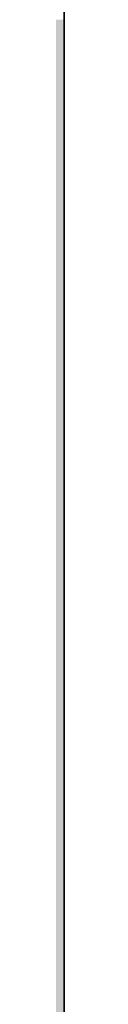
# Model space of a CAD drawing. Units: inches. Extents: x 2091 to 2899, y 967 to 2217.
# Tile 157 of 256: x 2212 to 2212, y 1131 to 1152. Entities that reach past the tile are written whole.
import ezdxf

# ---------------------------------------------------------------- set-up
doc = ezdxf.new("R2010")
doc.units = ezdxf.units.IN
doc.layers.add('A-WALL', color=7, linetype='Continuous', lineweight=35)
doc.layers.add('A-WALL-PATT', color=141, linetype='Continuous', lineweight=13, true_color=0xadddf7)

msp = doc.modelspace()

# ---------------------------------------------------------------- hatches: boundary and pattern name
at = {"layer": 'A-WALL-PATT'}
h = msp.add_hatch(color=256, dxfattribs=at)
h.dxf.hatch_style = 1
h.paths.add_polyline_path([(2212.144, 1941.419), (2387.644, 1941.419), (2387.644, 1824.419), (2392.144, 1824.419), (2392.144, 1941.419), (2609.644, 1941.419), (2609.644, 1825.919), (2614.144, 1825.919), (2614.144, 1941.419), (2794.144, 1941.419), (2794.144, 1928.762), (2803.144, 1928.762), (2803.144, 2050.919), (2203.144, 2050.919), (2203.144, 1900.758), (2212.144, 1900.758)])
h.paths.add_polyline_path([(2212.144, 1945.919), (2212.144, 2041.919), (2794.144, 2041.919), (2794.144, 1945.919), (2402.248, 1945.919), (2401.102, 1945.776), (2398.702, 1945.776)], flags=16)
h.paths.add_polyline_path([(2230.23, 1948.063), (2227.35, 1949.503), (2225.91, 1951.903), (2223.99, 1952.863), (2223.03, 1955.263), (2222.07, 1959.583), (2222.07, 1963.423), (2223.03, 1965.663), (2223.99, 1965.343), (2225.586, 1963.861), (2226.912, 1964.957), (2226.949, 1965.939), (2227.778, 1966.952), (2228.2, 1968.879), (2230.71, 1964.863), (2233.59, 1966.303), (2233.607, 1966.332), (2233.773, 1964.938), (2234.634, 1963.676), (2235.03, 1963.903), (2236.282, 1965.572), (2235.99, 1962.943), (2237.955, 1957.54), (2238.39, 1957.903), (2239.216, 1960.306), (2238.655, 1966.385), (2238.693, 1966.438), (2238.841, 1967.5), (2238.78, 1967.687), (2238.881, 1967.787), (2238.667, 1966.252), (2239.216, 1960.306), (2238.39, 1957.903), (2236.95, 1956.703), (2234.55, 1949.983)], flags=0)
h.paths.add_polyline_path([(2278.012, 1948.063), (2276.496, 1947.873), (2275.85, 1947.689), (2274.652, 1947.103)], flags=0)
h.paths.add_polyline_path([(2269.852, 1955.743), (2268.276, 1956.629), (2270.867, 1956.348), (2269.372, 1958.143), (2268.715, 1959.192), (2270.57, 1958.729), (2268.581, 1961.906), (2270.812, 1960.892), (2270.812, 1963.423), (2271.393, 1964.779), (2270.292, 1966.156), (2271.772, 1965.663), (2272.141, 1966.525), (2273.93, 1965.929), (2275.63, 1968.054), (2276.332, 1966.722), (2276.52, 1966.952), (2276.942, 1968.879), (2277.734, 1967.611), (2278.14, 1969.465), (2279.659, 1967.034), (2280.412, 1966.783), (2280.949, 1967.589), (2281.61, 1967.369), (2282.133, 1968.154), (2282.349, 1966.333), (2282.35, 1966.333), (2283.408, 1968.095), (2283.713, 1965.524), (2284.32, 1964.634), (2284.512, 1964.889), (2284.235, 1965.705), (2284.5, 1967.319), (2284.908, 1965.417), (2285.396, 1966.069), (2285.433, 1966.291), (2285.473, 1966.171), (2286.354, 1967.345), (2286.222, 1966.158), (2287.663, 1968.08), (2287.714, 1968.443), (2288.482, 1969.017), (2288.574, 1968.729), (2288.917, 1969.069), (2288.607, 1966.838), (2288.929, 1963.351), (2288.935, 1963.357), (2288.93, 1963.34), (2289.015, 1962.414), (2290.111, 1963.875), (2290.133, 1963.943), (2290.218, 1964.017), (2290.111, 1963.875), (2289.156, 1960.892), (2288.594, 1959.257), (2288.572, 1959.103), (2289.532, 1960.543), (2290.012, 1962.463), (2290.192, 1962.643), (2289.77, 1959.689), (2286.89, 1957.289), (2284.49, 1950.569), (2283.315, 1950.046), (2283.292, 1949.983), (2280.29, 1948.649), (2281.13, 1948.649), (2282.57, 1948.169), (2283.205, 1948.063), (2278.972, 1948.063), (2276.092, 1949.503), (2274.652, 1951.903), (2272.732, 1952.863)], flags=0)
h.paths.add_polyline_path([(2271.159, 1958.022), (2272.97, 1955.849), (2272.01, 1960.169), (2272.01, 1964.009), (2272.624, 1965.443), (2274.328, 1963.861), (2275.654, 1964.957), (2275.638, 1964.539), (2277.412, 1966.007), (2277.033, 1965.157), (2276.83, 1964.976), (2276.766, 1963.295), (2277.45, 1962.66), (2279.452, 1964.863), (2282.332, 1966.303), (2283.53, 1966.889), (2283.295, 1966.771), (2283.913, 1963.885), (2284.899, 1964.448), (2284.732, 1962.943), (2286.697, 1957.54), (2287.132, 1957.903), (2287.542, 1959.095), (2287.779, 1958.442), (2285.683, 1956.695), (2285.877, 1959.795), (2284.732, 1962.943), (2284.899, 1964.448), (2283.913, 1963.885), (2284.224, 1962.434), (2283.424, 1963.605), (2281.61, 1962.569), (2281.13, 1960.169), (2282.09, 1956.329), (2283.05, 1952.969), (2282.57, 1950.569), (2280.17, 1948.649), (2279.883, 1948.792), (2278.972, 1948.063), (2278.972, 1949.023), (2278.672, 1949.397), (2277.29, 1950.089), (2275.85, 1952.489), (2273.93, 1953.449), (2272.49, 1954.889), (2271.922, 1954.889), (2271.772, 1955.263)], flags=0)
h.paths.add_polyline_path([(2311.994, 1955.743), (2312.063, 1955.674), (2312.055, 1955.709)], flags=0)
h.paths.add_polyline_path([(2331.956, 1963.952), (2333.396, 1965.392), (2331.077, 1963.357), (2330.999, 1963.112)], flags=0)
h.paths.add_polyline_path([(2310.554, 1954.303), (2307.04, 1956.28), (2310.763, 1955.876), (2312.474, 1953.823), (2313.434, 1951.423), (2315.354, 1950.463), (2316.794, 1948.063), (2317.466, 1947.727), (2319.369, 1947.965), (2317.754, 1949.983), (2317.57, 1950.61), (2316.794, 1951.903), (2314.874, 1952.863), (2313.914, 1955.263), (2311.514, 1958.143), (2309.375, 1961.559), (2311.514, 1960.337), (2311.514, 1961.983), (2310.605, 1963.12), (2311.727, 1962.479), (2312.418, 1964.093), (2312.256, 1964.296), (2313.194, 1963.983), (2313.914, 1965.663), (2314.647, 1965.419), (2315.354, 1966.303), (2316.794, 1967.743), (2316.157, 1966.947), (2317.034, 1965.282), (2317.223, 1965.512), (2317.777, 1968.046), (2318.474, 1966.722), (2318.663, 1966.952), (2319.084, 1968.879), (2321.207, 1965.482), (2322.161, 1966.914), (2322.554, 1966.783), (2322.786, 1967.131), (2322.882, 1966.324), (2323.312, 1965.722), (2323.651, 1965.891), (2324.396, 1967.133), (2324.657, 1964.938), (2324.972, 1964.477), (2325.387, 1967.001), (2325.941, 1964.418), (2327.229, 1966.136), (2327.166, 1965.572), (2328.059, 1966.763), (2328.225, 1966.247), (2329.668, 1967.677), (2329.665, 1967.687), (2329.765, 1967.787), (2329.551, 1966.252), (2330.1, 1960.306), (2329.333, 1958.073), (2329.313, 1957.935), (2329.634, 1958.203), (2330.234, 1959.103), (2330.714, 1961.023), (2331.034, 1961.343), (2330.714, 1959.103), (2329.634, 1958.203), (2329.274, 1957.663), (2327.712, 1956.361), (2325.434, 1949.983), (2324.334, 1949.494), (2323.994, 1948.543), (2319.674, 1946.623), (2316.794, 1948.063), (2315.354, 1950.463), (2313.434, 1951.423)], flags=0)
h.paths.add_polyline_path([(2321.336, 1947.952), (2321.114, 1948.063), (2321.114, 1949.023), (2319.194, 1951.423), (2316.794, 1959.583), (2316.663, 1959.583), (2315.354, 1958.143), (2314.394, 1958.143), (2313.148, 1958.709), (2312.954, 1959.583), (2312.954, 1960.892), (2315.834, 1959.583), (2316.663, 1959.583), (2317.315, 1960.299), (2315.03, 1962.421), (2316.356, 1963.517), (2316.372, 1963.952), (2316.47, 1963.861), (2317.796, 1964.957), (2317.755, 1963.89), (2319.175, 1965.157), (2319.498, 1965.881), (2321.114, 1965.343), (2323.236, 1962.372), (2325.686, 1963.773), (2325.543, 1962.481), (2325.199, 1963.494), (2324.479, 1963.082), (2324.926, 1960.994), (2324.078, 1962.236), (2322.415, 1961.286), (2322.074, 1959.583), (2323.034, 1955.743), (2323.994, 1952.383), (2323.514, 1949.983), (2322.143, 1948.886), (2322.074, 1948.543)], flags=0)
h.paths.add_polyline_path([(2320.207, 1963.337), (2320.154, 1963.423), (2320.394, 1963.543)], flags=0)
h.paths.add_polyline_path([(2353.851, 1965.811), (2354.031, 1965.751), (2354.331, 1966.451), (2354.331, 1966.931)], flags=0)
h.paths.add_polyline_path([(2359.021, 1969.026), (2359.098, 1968.902), (2359.234, 1969.52), (2359.234, 1970)], flags=0)
h.paths.add_polyline_path([(2358.257, 1966.682), (2357.984, 1966.348), (2358.211, 1966.146), (2358.41, 1966.39)], flags=0)
h.paths.add_polyline_path([(2357.768, 1966.059), (2357.732, 1965.105), (2357.751, 1965.121), (2357.77, 1965.607), (2357.77, 1966.058)], flags=0)
h.paths.add_polyline_path([(2359.112, 1965.305), (2359.112, 1964.825), (2359.845, 1966.468), (2359.845, 1966.948)], flags=0)
h.paths.add_polyline_path([(2360.224, 1966.621), (2360.699, 1969.363), (2360.699, 1969.843), (2360.211, 1967.026), (2360.211, 1966.643)], flags=0)
h.paths.add_polyline_path([(2363.451, 1967.891), (2363.451, 1968.371), (2362.491, 1966.931), (2362.656, 1966.699)], flags=0)
h.paths.add_polyline_path([(2364.476, 1966.079), (2365.851, 1968.371), (2365.851, 1968.851), (2364.428, 1966.48)], flags=0)
h.paths.add_polyline_path([(2366.314, 1965.853), (2366.367, 1965.696), (2366.803, 1968.346), (2366.803, 1968.826)], flags=0)
h.paths.add_polyline_path([(2367.165, 1965.804), (2367.291, 1966.931), (2367.291, 1967.411), (2367.103, 1965.72)], flags=0)
h.paths.add_polyline_path([(2370.037, 1959.974), (2371.014, 1963.025), (2371.014, 1963.505), (2370.037, 1960.454)], flags=0)
h.paths.add_polyline_path([(2371.611, 1960.211), (2372.571, 1961.651), (2372.571, 1962.131), (2371.803, 1960.979)], flags=0)
h.paths.add_polyline_path([(2350.874, 1956.005), (2351.931, 1955.891), (2354.491, 1953.331), (2353.851, 1954.931), (2351.451, 1957.811), (2347.936, 1963.426), (2347.936, 1963.906), (2351.451, 1958.291), (2353.705, 1955.585), (2352.891, 1959.251), (2352.891, 1959.731), (2352.891, 1961.925), (2356.731, 1959.731), (2358.454, 1961.627), (2354.811, 1965.011), (2355.031, 1965.286), (2358.691, 1961.887), (2361.531, 1965.011), (2364.376, 1966.433), (2364.524, 1965.187), (2365.454, 1963.824), (2365.881, 1964.068), (2365.371, 1966.451), (2365.371, 1966.931), (2366.811, 1960.211), (2366.811, 1959.731), (2366.389, 1952.981), (2367.771, 1956.851), (2368.641, 1957.576), (2366.811, 1962.611), (2366.811, 1963.091), (2368.775, 1957.688), (2369.211, 1958.051), (2370.002, 1960.352), (2369.475, 1966.053), (2369.513, 1966.106), (2369.514, 1966.111), (2369.475, 1966.533), (2369.513, 1966.586), (2369.615, 1967.313), (2369.183, 1968.659), (2369.183, 1969.139), (2369.601, 1967.835), (2369.701, 1967.934), (2369.718, 1968.055), (2370.145, 1968.374), (2369.779, 1968.011), (2369.701, 1967.454), (2370.468, 1968.214), (2369.675, 1967.266), (2369.514, 1966.111), (2370.037, 1960.454), (2370.037, 1959.974), (2369.442, 1958.243), (2370.651, 1959.251), (2371.046, 1962.018), (2371.131, 1962.131), (2370.651, 1958.771), (2367.771, 1956.371), (2365.371, 1949.651), (2362.079, 1948.188), (2363.451, 1947.731), (2361.051, 1947.731), (2360.091, 1947.731), (2357.104, 1947.357), (2360.091, 1948.211), (2358.171, 1949.171), (2356.731, 1951.571), (2354.811, 1952.531), (2351.931, 1955.411)], flags=0)
h.paths.add_polyline_path([(2361.051, 1948.691), (2359.131, 1951.091), (2356.731, 1959.251), (2355.771, 1959.251), (2352.891, 1960.56), (2352.891, 1961.445), (2355.891, 1959.731), (2356.731, 1959.731), (2356.837, 1959.368), (2361.531, 1964.531), (2363.248, 1965.389), (2364.925, 1963.042), (2362.491, 1961.651), (2362.064, 1959.517), (2362.971, 1955.891), (2363.931, 1952.531), (2363.931, 1952.051), (2363.451, 1949.651), (2361.051, 1947.731)], flags=0)
h.paths.add_polyline_path([(2359.131, 1951.571), (2359.291, 1951.371), (2361.051, 1954.451), (2361.051, 1954.931)], flags=0)
h.paths.add_polyline_path([(2357.22, 1966.546), (2356.793, 1968.815), (2356.793, 1969.295), (2357.22, 1967.026)], flags=0)
h.paths.add_polyline_path([(2361.051, 1954.451), (2361.531, 1958.771), (2361.531, 1959.251), (2361.051, 1954.931)], flags=0)
h.paths.add_polyline_path([(2402.548, 1948.486), (2402.302, 1948.416), (2402.59, 1948.416)], flags=0)
h.paths.add_polyline_path([(2394.142, 1956.096), (2395.685, 1954.553), (2396.72, 1953.971), (2396.062, 1955.616), (2395.241, 1956.601), (2395.879, 1956.442), (2395.102, 1959.936), (2395.102, 1963.776), (2396.062, 1966.016), (2397.022, 1965.696), (2398.618, 1964.214), (2399.944, 1965.31), (2399.981, 1966.292), (2400.811, 1967.305), (2401.232, 1969.232), (2403.538, 1965.543), (2403.942, 1967.389), (2404.702, 1967.136), (2405.46, 1966.075), (2406.622, 1966.656), (2406.64, 1966.685), (2406.805, 1965.291), (2406.926, 1965.115), (2407.342, 1964.976), (2407.874, 1965.774), (2408.169, 1964.398), (2409.315, 1965.925), (2409.217, 1965.051), (2409.445, 1963.131), (2410.306, 1961.87), (2410.702, 1962.096), (2411.442, 1963.082), (2411.165, 1963.898), (2411.616, 1966.64), (2411.725, 1966.791), (2411.873, 1967.853), (2411.813, 1968.041), (2411.913, 1968.14), (2411.699, 1966.605), (2412.248, 1960.659), (2413.225, 1963.71), (2414.378, 1964.721), (2414.513, 1965.693), (2414.453, 1965.881), (2414.553, 1965.98), (2414.378, 1964.721), (2414.52, 1964.846), (2414.365, 1964.631), (2414.339, 1964.445), (2414.888, 1958.499), (2414.062, 1956.096), (2412.622, 1954.896), (2410.171, 1948.033), (2410.017, 1948.084), (2405.902, 1946.256), (2405.902, 1947.216), (2405.204, 1948.089), (2404.222, 1948.416), (2403.262, 1948.416), (2400.382, 1949.856), (2399.662, 1951.056), (2397.982, 1952.736), (2397.022, 1953.216), (2395.685, 1954.553), (2392.657, 1956.257)], flags=0)
h.paths.add_polyline_path([(2409.086, 1964.407), (2409.13, 1964.276), (2409.262, 1964.496)], flags=0)
h.paths.add_polyline_path([(2397.742, 1961.616), (2398.702, 1963.856), (2399.662, 1963.536), (2401.427, 1965.741), (2401.791, 1966.559), (2402.071, 1965.071), (2402.836, 1964.393), (2403.262, 1964.915), (2403.338, 1964.771), (2402.616, 1963.976), (2402.499, 1960.902), (2403.543, 1959.932), (2404.413, 1960.89), (2404.702, 1962.336), (2407.916, 1964.172), (2409.52, 1961.927), (2410.987, 1957.893), (2411.422, 1958.256), (2412.048, 1960.076), (2412.41, 1959.079), (2411.676, 1958.467), (2411.662, 1958.256), (2411.626, 1958.426), (2409.982, 1957.056), (2407.582, 1950.336), (2403.262, 1948.416), (2403.262, 1949.376), (2401.342, 1951.776), (2399.417, 1958.324), (2397.742, 1959.085), (2397.742, 1959.97), (2397.102, 1960.336), (2397.742, 1960.045)], flags=0)
h.paths.add_polyline_path([(2405.902, 1952.976), (2405.95, 1953.408), (2406.017, 1953.176)], flags=0)
h.paths.add_polyline_path([(2449.818, 1967.114), (2449.752, 1967.136), (2449.794, 1967.078)], flags=0)
h.paths.add_polyline_path([(2451.698, 1966.618), (2451.741, 1966.69), (2451.692, 1966.666)], flags=0)
h.paths.add_polyline_path([(2454.344, 1965.738), (2455.752, 1967.616), (2455.992, 1968.096), (2454.364, 1965.925)], flags=0)
h.paths.add_polyline_path([(2457.547, 1968.864), (2457.787, 1969.344), (2457.054, 1968.796), (2457.008, 1968.46)], flags=0)
h.paths.add_polyline_path([(2456.922, 1967.857), (2456.802, 1968.229), (2456.723, 1967.66)], flags=0)
h.paths.add_polyline_path([(2457.302, 1967.377), (2457.542, 1967.857), (2456.81, 1966.84), (2456.741, 1966.7), (2456.749, 1966.608)], flags=0)
h.paths.add_polyline_path([(2458.275, 1963.71), (2458.155, 1963.335), (2460.354, 1965.265), (2460.594, 1965.745)], flags=0)
h.paths.add_polyline_path([(2458.392, 1962.816), (2458.364, 1962.618), (2459.592, 1964.256), (2459.832, 1964.736)], flags=0)
h.paths.add_polyline_path([(2459.352, 1962.816), (2459.272, 1962.496), (2460.072, 1963.296), (2460.312, 1963.776)], flags=0)
h.paths.add_polyline_path([(2458.68, 1960.608), (2458.632, 1960.416), (2459.592, 1961.856), (2459.832, 1962.336)], flags=0)
h.paths.add_polyline_path([(2437.838, 1956.243), (2439.192, 1956.096), (2441.352, 1953.936), (2440.872, 1955.136), (2438.472, 1958.016), (2438.072, 1958.656), (2438.712, 1958.496), (2440.64, 1956.183), (2439.912, 1959.456), (2439.912, 1963.296), (2441.352, 1966.656), (2441.592, 1967.136), (2441.112, 1966.016), (2442.072, 1965.696), (2443.989, 1968.092), (2444.241, 1966.751), (2444.917, 1966.152), (2445.677, 1967.08), (2446.255, 1969.725), (2446.495, 1970.205), (2446.282, 1969.232), (2447.363, 1967.503), (2447.72, 1969.568), (2447.96, 1970.048), (2447.485, 1967.307), (2448.792, 1965.216), (2448.472, 1964.864), (2448.552, 1964.736), (2451.452, 1966.186), (2451.615, 1964.811), (2452.308, 1963.796), (2453.235, 1964.326), (2454.072, 1960.416), (2453.629, 1953.318), (2454.792, 1956.576), (2455.032, 1957.056), (2455.719, 1957.628), (2453.832, 1962.816), (2453.941, 1963.794), (2453.335, 1965.578), (2453.824, 1968.551), (2454.064, 1969.031), (2453.575, 1966.058), (2454.04, 1964.688), (2453.832, 1962.816), (2455.719, 1957.628), (2456.367, 1958.168), (2457.058, 1960.179), (2457.298, 1960.659), (2456.472, 1958.256), (2457.718, 1959.294), (2457.672, 1958.976), (2454.89, 1956.657), (2453.614, 1953.085), (2453.592, 1952.736), (2453.352, 1952.256), (2453.36, 1952.372), (2452.632, 1950.336), (2452.392, 1949.856), (2449.204, 1948.439), (2450.712, 1947.936), (2448.072, 1947.936), (2447.112, 1947.936), (2444.552, 1947.616), (2447.2, 1948.372), (2445.192, 1949.376), (2443.752, 1951.776), (2441.832, 1952.736), (2438.952, 1955.616)], flags=0)
h.paths.add_polyline_path([(2443.992, 1959.936), (2444.04, 1959.773), (2444.122, 1959.862)], flags=0)
h.paths.add_polyline_path([(2442.912, 1959.936), (2443.032, 1959.936), (2442.446, 1960.202)], flags=0)
h.paths.add_polyline_path([(2444.983, 1965.02), (2445.279, 1965.265), (2445.519, 1965.745), (2444.994, 1965.31)], flags=0)
h.paths.add_polyline_path([(2446.133, 1965.03), (2446.33, 1965.471), (2444.97, 1964.258), (2444.73, 1963.778)], flags=0)
h.paths.add_polyline_path([(2442.792, 1959.456), (2443.752, 1959.456), (2446.152, 1951.296), (2446.412, 1951.751), (2446.392, 1951.776), (2448.081, 1954.73), (2448.552, 1958.976), (2441.832, 1965.216), (2442.155, 1965.619), (2448.792, 1959.456), (2448.312, 1955.136), (2448.072, 1954.656), (2446.412, 1951.751), (2448.312, 1949.376), (2448.312, 1948.416), (2450.541, 1950.199), (2450.952, 1952.256), (2449.992, 1955.616), (2449.032, 1959.456), (2449.512, 1961.856), (2449.752, 1962.336), (2449.675, 1961.949), (2452.995, 1963.846), (2453.064, 1963.519), (2452.885, 1963.783), (2449.675, 1961.949), (2449.272, 1959.936), (2450.232, 1956.096), (2451.192, 1952.736), (2450.712, 1950.336), (2450.472, 1949.856), (2448.072, 1947.936), (2448.072, 1948.536), (2445.432, 1949.856), (2443.992, 1952.256), (2442.072, 1953.216), (2441.112, 1955.616), (2440.152, 1959.936), (2440.152, 1960.656)], flags=0)
h.paths.add_polyline_path([(2456.692, 1966.986), (2457.608, 1968.081), (2457.848, 1968.561), (2456.932, 1967.466)], flags=0)
h.paths.add_polyline_path([(2489.897, 1966.58), (2489.943, 1966.189), (2490.747, 1967.53), (2491.319, 1968.951)], flags=0)
h.paths.add_polyline_path([(2473.562, 1956.407), (2477.14, 1956.019), (2476.955, 1956.241), (2475.108, 1957.28), (2476.347, 1956.97), (2475.187, 1958.824), (2476.919, 1958.391), (2475.412, 1960.799), (2477.787, 1959.719), (2477.787, 1962.25), (2477.637, 1962.438), (2477.823, 1962.332), (2478.359, 1963.584), (2478.359, 1963.671), (2477.324, 1964.965), (2478.715, 1964.501), (2479.319, 1965.911), (2480.279, 1965.591), (2481.784, 1967.472), (2482.116, 1965.705), (2482.881, 1965.028), (2483.209, 1965.429), (2483.22, 1965.715), (2483.076, 1965.989), (2483.712, 1966.766), (2484.13, 1968.679), (2484.702, 1970.1), (2484.489, 1969.127), (2486.503, 1965.905), (2487.387, 1965.61), (2488.153, 1966.759), (2488.717, 1965.97), (2489.2, 1966.212), (2489.331, 1965.111), (2490.394, 1963.622), (2490.661, 1963.775), (2490.494, 1964.554), (2490.923, 1963.925), (2491.319, 1964.151), (2491.333, 1964.17), (2491.21, 1964.532), (2491.282, 1964.966), (2491.426, 1964.293), (2494.076, 1967.828), (2494.498, 1966.515), (2494.598, 1966.614), (2494.689, 1967.27), (2495.107, 1967.582), (2495.13, 1967.748), (2495.07, 1967.936), (2495.17, 1968.035), (2495.032, 1967.044), (2495.754, 1967.759), (2494.982, 1966.686), (2494.956, 1966.5), (2495.479, 1960.837), (2495.91, 1962.184), (2496.482, 1963.605), (2496.073, 1962.327), (2496.769, 1962.938), (2496.599, 1962.711), (2496.119, 1959.351), (2496.733, 1960.272), (2496.987, 1961.29), (2497.559, 1962.711), (2497.079, 1960.791), (2496.507, 1959.37), (2495.547, 1957.93), (2492.759, 1955.606), (2490.839, 1950.231), (2490.267, 1948.81), (2485.947, 1946.89), (2483.067, 1948.33), (2481.627, 1950.73), (2479.707, 1951.69), (2476.827, 1954.57)], flags=0)
h.paths.add_polyline_path([(2485.577, 1948.313), (2485.559, 1948.311), (2485.579, 1948.311)], flags=0)
h.paths.add_polyline_path([(2478.645, 1954.551), (2478.109, 1956.963), (2479.319, 1955.511), (2480.279, 1953.111), (2482.199, 1952.151), (2483.639, 1949.751), (2486.519, 1948.311), (2486.519, 1949.271), (2484.739, 1951.496), (2484.027, 1950.25), (2481.627, 1958.41), (2482.375, 1959.233), (2482.199, 1959.831), (2483.198, 1960.929), (2479.707, 1964.17), (2480.603, 1965.29), (2481.875, 1964.109), (2482.666, 1964.764), (2482.615, 1963.422), (2482.989, 1963.075), (2484.008, 1963.984), (2484.684, 1965.498), (2484.58, 1965.405), (2485.357, 1967.147), (2485.121, 1965.781), (2486.427, 1963.69), (2488.145, 1964.549), (2489.822, 1962.202), (2490.747, 1962.73), (2492, 1964.4), (2492.076, 1965.087), (2492.213, 1964.684), (2492.485, 1965.047), (2492.279, 1963.191), (2494.244, 1957.788), (2494.563, 1958.054), (2494.933, 1959.133), (2495.505, 1960.554), (2494.679, 1958.151), (2494.107, 1956.73), (2494.563, 1958.054), (2493.409, 1957.092), (2491.707, 1961.77), (2492, 1964.4), (2490.747, 1962.73), (2487.712, 1960.996), (2487.479, 1959.831), (2488.439, 1955.991), (2489.399, 1952.631), (2488.919, 1950.231), (2488.577, 1949.957), (2488.347, 1948.81), (2487.652, 1948.254), (2487.479, 1948.311), (2486.519, 1948.311), (2483.639, 1949.751), (2482.199, 1952.151), (2480.279, 1953.111), (2478.839, 1954.551)], flags=0)
h.paths.add_polyline_path([(2526.648, 1966.988), (2526.517, 1967.031), (2526.6, 1966.915)], flags=0)
h.paths.add_polyline_path([(2528.471, 1966.447), (2528.574, 1966.62), (2528.457, 1966.561)], flags=0)
h.paths.add_polyline_path([(2534.133, 1967.496), (2534.157, 1967.543), (2534.06, 1967.408)], flags=0)
h.paths.add_polyline_path([(2536.162, 1964.051), (2535.157, 1962.711), (2535.101, 1962.316), (2536.117, 1963.671), (2536.421, 1964.278)], flags=0)
h.paths.add_polyline_path([(2535.157, 1959.831), (2536.117, 1961.271), (2536.597, 1962.231), (2535.253, 1960.215)], flags=0)
h.paths.add_polyline_path([(2513.249, 1956.285), (2516.221, 1955.963), (2514.997, 1957.431), (2514.196, 1958.712), (2515.477, 1958.391), (2516.932, 1956.646), (2516.437, 1958.871), (2516.437, 1962.711), (2516.873, 1963.727), (2515.346, 1965.635), (2517.397, 1964.951), (2517.877, 1966.071), (2518.357, 1967.031), (2517.877, 1965.911), (2518.837, 1965.591), (2520.487, 1967.653), (2520.766, 1966.166), (2521.53, 1965.489), (2521.781, 1965.795), (2521.801, 1966.307), (2521.478, 1966.921), (2521.246, 1967.126), (2521.178, 1967.491), (2521.478, 1966.921), (2522.01, 1966.449), (2522.257, 1966.75), (2522.78, 1969.14), (2523.26, 1970.1), (2523.047, 1969.127), (2524.673, 1966.526), (2526.037, 1966.071), (2526.795, 1965.01), (2527.977, 1965.601), (2528.14, 1964.227), (2528.665, 1963.458), (2529.389, 1963.872), (2529.33, 1964.147), (2529.481, 1963.925), (2529.877, 1964.151), (2529.984, 1964.293), (2529.789, 1965.203), (2530.062, 1964.398), (2532.802, 1968.051), (2533.148, 1966.976), (2533.248, 1967.075), (2533.339, 1967.731), (2533.673, 1967.98), (2533.728, 1968.035), (2533.514, 1966.5), (2534.025, 1960.972), (2534.56, 1962.645), (2535.04, 1963.605), (2534.063, 1960.554), (2533.237, 1958.151), (2534.288, 1959.027), (2534.197, 1958.391), (2531.513, 1956.154), (2529.397, 1950.231), (2528.917, 1949.271), (2526.449, 1948.174), (2527.477, 1947.831), (2530.357, 1947.351), (2524.597, 1947.351), (2521.717, 1948.791), (2520.277, 1951.191), (2518.357, 1952.151), (2515.477, 1955.031)], flags=0)
h.paths.add_polyline_path([(2523.935, 1967.19), (2523.62, 1966.484), (2523.77, 1966.242)], flags=0)
h.paths.add_polyline_path([(2518.837, 1953.111), (2517.877, 1955.511), (2516.885, 1959.977), (2516.917, 1959.962), (2516.917, 1962.025), (2520.757, 1959.831), (2522.025, 1961.226), (2518.357, 1964.631), (2519.003, 1965.438), (2520.433, 1964.109), (2521.301, 1964.827), (2521.245, 1963.355), (2525.638, 1959.276), (2526.037, 1961.271), (2529.397, 1963.191), (2530.65, 1964.861), (2530.665, 1964.998), (2530.692, 1964.917), (2531.088, 1965.445), (2530.946, 1964.169), (2530.692, 1964.917), (2529.397, 1963.191), (2526.363, 1961.457), (2526.037, 1959.831), (2526.997, 1955.991), (2527.957, 1952.631), (2527.477, 1950.231), (2527.134, 1949.957), (2526.974, 1949.154), (2526.697, 1949.031), (2524.597, 1947.351), (2524.597, 1948.311), (2524.277, 1948.711), (2522.197, 1949.751), (2520.757, 1952.151)], flags=0)
h.paths.add_polyline_path([(2520.277, 1958.871), (2520.853, 1959.505), (2523.157, 1951.671), (2524.614, 1954.22), (2524.597, 1954.071), (2522.677, 1950.711)], flags=0)
h.paths.add_polyline_path([(2559.371, 1966.311), (2559.398, 1966.325), (2559.402, 1966.345)], flags=0)
h.paths.add_polyline_path([(2549.771, 1957.191), (2552.651, 1954.311), (2552.134, 1955.603), (2550.611, 1957.431), (2547.096, 1963.046), (2545.776, 1965.206), (2549.291, 1959.591), (2551.691, 1956.711), (2550.793, 1960.752), (2550.731, 1960.78), (2550.731, 1964.871), (2551.691, 1967.111), (2552.651, 1966.791), (2554.247, 1965.309), (2555.034, 1965.96), (2555.582, 1966.645), (2555.61, 1967.387), (2556.439, 1968.401), (2556.861, 1970.327), (2559.371, 1966.311), (2560.691, 1964.151), (2562.409, 1965.01), (2561.651, 1966.071), (2560.331, 1968.231), (2561.758, 1966.233), (2562.347, 1967.116), (2562.434, 1966.387), (2563.128, 1965.37), (2563.571, 1965.591), (2563.588, 1965.62), (2563.363, 1967.524), (2563.722, 1965.844), (2565.06, 1968.073), (2564.733, 1965.129), (2565.118, 1963.333), (2567.445, 1966.436), (2567.316, 1967.833), (2567.354, 1967.886), (2567.502, 1968.948), (2567.441, 1969.136), (2567.542, 1969.235), (2567.328, 1967.7), (2567.877, 1961.754), (2568.747, 1964.47), (2568.636, 1965.673), (2568.674, 1965.726), (2568.822, 1966.788), (2568.761, 1966.976), (2568.862, 1967.075), (2568.648, 1965.54), (2568.726, 1964.693), (2568.854, 1964.805), (2568.747, 1964.47), (2568.817, 1963.706), (2568.971, 1963.911), (2568.866, 1963.177), (2569.197, 1959.594), (2568.371, 1957.191), (2566.931, 1955.991), (2564.62, 1949.521), (2564.651, 1949.511), (2564.617, 1949.511), (2564.531, 1949.271), (2560.211, 1947.351), (2557.331, 1948.791), (2556.045, 1950.934), (2556.011, 1950.951), (2555.857, 1951.208), (2553.971, 1952.151), (2551.091, 1955.031), (2546.65, 1957.53)], flags=0)
h.paths.add_polyline_path([(2567.026, 1959.33), (2567.035, 1959.305), (2567.051, 1959.351)], flags=0)
h.paths.add_polyline_path([(2551.968, 1962.518), (2553.011, 1964.951), (2553.971, 1964.631), (2555.567, 1963.149), (2556.893, 1964.246), (2556.93, 1965.227), (2557.144, 1965.489), (2556.42, 1966.131), (2556.391, 1966.105), (2556.38, 1966.166), (2556.42, 1966.131), (2556.952, 1966.605), (2557.092, 1966.919), (2557.571, 1966.01), (2557.759, 1966.241), (2557.418, 1964.68), (2556.893, 1964.246), (2556.807, 1961.998), (2560.691, 1958.391), (2560.636, 1957.893), (2560.811, 1957.191), (2561.771, 1953.831), (2561.291, 1951.431), (2559.11, 1949.687), (2559.156, 1949.629), (2563.027, 1951.349), (2562.611, 1949.271), (2560.211, 1947.351), (2560.211, 1948.311), (2559.251, 1949.511), (2558.891, 1949.511), (2558.891, 1949.961), (2558.291, 1950.711), (2558.054, 1951.518), (2556.971, 1952.871), (2555.068, 1959.341), (2552.051, 1961.065), (2552.051, 1962.471)], flags=0)
h.paths.add_polyline_path([(2588.33, 1958.391), (2588.61, 1958.111), (2588.553, 1958.367)], flags=0)
h.paths.add_polyline_path([(2594.745, 1950.493), (2593.958, 1953.172), (2593.13, 1954.551), (2591.21, 1955.511), (2590.25, 1957.911), (2588.309, 1960.24), (2586.177, 1961.209), (2587.85, 1960.791), (2587.253, 1961.744), (2588.441, 1961.065), (2588.441, 1962.656), (2588.422, 1962.665), (2588.441, 1962.711), (2586.914, 1964.62), (2588.877, 1963.728), (2589.29, 1964.692), (2589.29, 1966.071), (2590.25, 1968.311), (2591.21, 1967.991), (2592.806, 1966.509), (2594.132, 1967.606), (2594.169, 1968.587), (2594.999, 1969.601), (2595.42, 1971.527), (2597.93, 1967.511), (2600.81, 1968.951), (2600.827, 1968.98), (2600.993, 1967.587), (2601.854, 1966.325), (2602.107, 1966.47), (2602.236, 1967.255), (2602.357, 1966.693), (2603.502, 1968.221), (2603.21, 1965.591), (2605.175, 1960.188), (2605.507, 1960.465), (2605.026, 1965.673), (2605.064, 1965.726), (2605.212, 1966.788), (2605.152, 1966.976), (2605.252, 1967.075), (2605.343, 1967.731), (2605.953, 1968.187), (2605.875, 1969.033), (2605.913, 1969.086), (2606.061, 1970.148), (2606, 1970.336), (2606.101, 1970.435), (2605.887, 1968.9), (2606.436, 1962.954), (2605.61, 1960.551), (2605.997, 1960.874), (2606.564, 1962.645), (2608.241, 1964.117), (2608.01, 1963.191), (2607.05, 1961.751), (2606.631, 1961.402), (2606.201, 1958.391), (2603.321, 1955.991), (2600.921, 1949.271), (2596.601, 1947.351), (2593.721, 1948.791), (2592.857, 1950.231), (2592.65, 1950.231)], flags=0)
h.paths.add_polyline_path([(2596.601, 1947.351), (2596.601, 1948.311), (2594.681, 1950.711), (2596.155, 1953.29), (2595.53, 1954.071), (2593.199, 1961.996), (2592.651, 1962.505), (2591.78, 1963.003), (2593.283, 1964.246), (2593.32, 1965.227), (2594.15, 1966.241), (2594.571, 1968.167), (2596.183, 1965.589), (2596.951, 1966.435), (2598.041, 1966.071), (2598.799, 1965.01), (2599.961, 1965.591), (2599.979, 1965.62), (2600.144, 1964.227), (2601.005, 1962.965), (2601.401, 1963.191), (2602.653, 1964.861), (2602.361, 1962.231), (2603.793, 1958.295), (2601.978, 1953.212), (2601.946, 1952.709), (2599.469, 1951.608), (2599.001, 1949.271)], flags=0)
h.paths.add_polyline_path([(2597.561, 1958.871), (2597.671, 1959.419), (2597.595, 1958.736)], flags=0)
h.paths.add_polyline_path([(2623.666, 1961.254), (2625.519, 1960.791), (2624.966, 1961.676), (2627.199, 1960.66), (2627.199, 1961.151), (2626.959, 1962.231), (2626.959, 1963.491), (2625.582, 1965.212), (2626.959, 1964.425), (2626.959, 1965.831), (2626.869, 1965.861), (2627.919, 1968.311), (2628.879, 1967.991), (2630.475, 1966.509), (2631.801, 1967.606), (2631.838, 1968.587), (2632.668, 1969.601), (2633.089, 1971.527), (2635.599, 1967.511), (2638.479, 1968.951), (2638.497, 1968.98), (2638.662, 1967.587), (2639.176, 1966.833), (2639.78, 1967.84), (2640.026, 1966.693), (2641.171, 1968.221), (2640.879, 1965.591), (2641.114, 1964.945), (2641.411, 1965.341), (2641.308, 1964.412), (2642.844, 1960.188), (2643.279, 1960.551), (2644.085, 1962.895), (2643.784, 1966.153), (2643.807, 1966.185), (2643.601, 1968.418), (2643.523, 1968.661), (2643.73, 1970.148), (2643.67, 1970.336), (2643.77, 1970.435), (2643.556, 1968.9), (2643.601, 1968.418), (2643.91, 1967.456), (2644.01, 1967.555), (2643.812, 1966.132), (2644.105, 1962.954), (2644.239, 1961.351), (2644.719, 1961.751), (2645.033, 1962.222), (2645.322, 1963.125), (2646.076, 1963.787), (2645.033, 1962.222), (2644.345, 1960.074), (2643.519, 1957.671), (2642.079, 1956.471), (2639.72, 1949.864), (2639.876, 1949.838), (2635.359, 1947.831), (2632.479, 1949.271), (2631.039, 1951.671), (2629.119, 1952.631), (2628.159, 1955.031), (2625.759, 1957.911)], flags=0)
h.paths.add_polyline_path([(2627.816, 1956.574), (2627.374, 1958.566), (2626.376, 1959.763), (2627.199, 1959.351), (2627.374, 1958.566), (2627.919, 1957.911), (2628.879, 1955.511), (2630.799, 1954.551), (2632.239, 1952.151), (2633.315, 1951.613), (2631.039, 1959.351), (2631.498, 1959.856), (2630.799, 1962.231), (2631.45, 1962.947), (2630.715, 1963.629), (2632.041, 1964.726), (2632.078, 1965.707), (2632.292, 1965.969), (2631.705, 1966.489), (2633.136, 1967.766), (2633.329, 1968.647), (2634.675, 1966.494), (2635.208, 1967.081), (2636.799, 1966.551), (2637.676, 1967.867), (2638.994, 1966.022), (2639.705, 1966.429), (2641.119, 1959.831), (2640.93, 1956.806), (2639.439, 1952.631), (2638.227, 1952.093), (2637.759, 1949.751), (2635.359, 1947.831), (2635.359, 1948.791), (2633.439, 1951.191), (2633.315, 1951.613), (2632.239, 1952.151), (2630.799, 1954.551), (2628.879, 1955.511)], flags=0)
h.paths.add_polyline_path([(2637.759, 1953.831), (2637.279, 1955.511), (2636.319, 1959.351), (2636.799, 1961.751), (2639.234, 1963.142), (2637.557, 1965.49), (2638.739, 1966.081), (2638.902, 1964.707), (2639.763, 1963.445), (2636.799, 1961.751), (2636.532, 1960.418), (2637.039, 1958.391), (2637.999, 1955.031)], flags=0)
h.paths.add_polyline_path([(2668.567, 1951.431), (2667.607, 1953.831), (2665.207, 1956.711), (2662.294, 1961.365), (2665.447, 1959.591), (2666.647, 1958.391), (2666.647, 1959.975), (2666.058, 1960.682), (2666.647, 1960.345), (2666.647, 1961.991), (2666.7, 1962.114), (2666.407, 1963.431), (2666.407, 1967.271), (2667.367, 1969.511), (2668.327, 1969.191), (2669.923, 1967.709), (2671.249, 1968.806), (2671.286, 1969.787), (2672.116, 1970.801), (2672.537, 1972.727), (2675.047, 1968.711), (2677.927, 1970.151), (2677.945, 1970.18), (2678.11, 1968.787), (2678.971, 1967.525), (2679.367, 1967.751), (2680.62, 1969.421), (2680.327, 1966.791), (2682.292, 1961.388), (2682.727, 1961.751), (2683.358, 1963.587), (2683.232, 1964.953), (2683.27, 1965.006), (2683.393, 1965.889), (2683.36, 1966.249), (2683.358, 1966.256), (2683.359, 1966.257), (2682.992, 1970.233), (2683.03, 1970.286), (2683.178, 1971.348), (2683.118, 1971.536), (2683.218, 1971.635), (2683.004, 1970.1), (2683.359, 1966.257), (2683.458, 1966.355), (2683.393, 1965.889), (2683.414, 1965.665), (2684.424, 1966.872), (2683.553, 1964.154), (2683.358, 1963.587), (2683.793, 1958.874), (2682.967, 1956.471), (2681.527, 1955.271), (2680.109, 1951.3), (2680.085, 1950.912), (2679.977, 1950.93), (2679.127, 1948.551), (2674.807, 1946.631), (2671.927, 1948.071), (2670.487, 1950.471)], flags=0)
h.paths.add_polyline_path([(2671.936, 1953.227), (2671.687, 1953.351), (2670.247, 1955.751), (2668.327, 1956.711), (2667.357, 1959.138), (2669.527, 1958.151), (2670.487, 1958.151), (2671.479, 1959.242), (2670.684, 1961.945), (2668.89, 1963.612), (2667.307, 1964.331), (2668.567, 1963.911), (2668.831, 1964.241), (2670.247, 1963.431), (2672.422, 1965.823), (2672.777, 1967.447), (2673.234, 1966.716), (2674.412, 1968.012), (2673.981, 1965.522), (2675.287, 1963.431), (2675.554, 1963.564), (2675.932, 1965.456), (2676.247, 1965.351), (2677.005, 1964.29), (2678.167, 1964.871), (2679.607, 1967.271), (2680.327, 1963.911), (2680.307, 1963.577), (2680.347, 1963.458), (2680.86, 1964.141), (2680.567, 1961.511), (2681.104, 1960.037), (2678.887, 1953.831), (2677.092, 1953.033), (2677.687, 1950.951), (2677.207, 1948.551), (2674.807, 1946.631), (2674.807, 1947.591), (2672.887, 1949.991)], flags=0)
h.paths.add_polyline_path([(2673.985, 1951.911), (2674.567, 1952.931), (2674.567, 1951.911), (2676.967, 1953.831), (2677.447, 1956.231), (2676.487, 1959.591), (2676.247, 1960.551), (2679.73, 1962.541), (2680.059, 1961.002), (2679.211, 1962.245), (2676.247, 1960.551), (2676.487, 1959.591), (2677.447, 1956.231), (2676.967, 1953.831), (2674.567, 1951.911)], flags=0)
h.paths.add_polyline_path([(2707.479, 1952.815), (2706.519, 1955.215), (2705.559, 1959.535), (2705.559, 1963.375), (2706.519, 1965.615), (2707.479, 1965.295), (2709.075, 1963.813), (2710.401, 1964.909), (2710.438, 1965.891), (2711.268, 1966.904), (2711.689, 1968.831), (2714.199, 1964.815), (2717.079, 1966.255), (2717.097, 1966.284), (2717.262, 1964.89), (2718.123, 1963.628), (2718.519, 1963.855), (2719.771, 1965.524), (2719.479, 1962.895), (2721.444, 1957.492), (2721.879, 1957.855), (2722.705, 1960.258), (2722.144, 1966.337), (2722.182, 1966.39), (2722.33, 1967.452), (2722.27, 1967.639), (2722.37, 1967.739), (2722.156, 1966.204), (2722.705, 1960.258), (2721.879, 1957.855), (2720.439, 1956.655), (2718.039, 1949.935), (2713.719, 1948.015), (2710.839, 1949.455), (2709.399, 1951.855)], flags=0)
h.paths.add_polyline_path([(2749.301, 1952.815), (2748.341, 1955.215), (2747.381, 1959.535), (2747.381, 1963.375), (2748.341, 1965.615), (2749.301, 1965.295), (2750.897, 1963.813), (2752.223, 1964.909), (2752.26, 1965.891), (2753.09, 1966.904), (2753.511, 1968.831), (2756.021, 1964.815), (2758.901, 1966.255), (2758.919, 1966.284), (2759.084, 1964.89), (2759.945, 1963.628), (2760.341, 1963.855), (2761.593, 1965.524), (2761.301, 1962.895), (2763.266, 1957.492), (2763.701, 1957.855), (2764.527, 1960.258), (2763.966, 1966.337), (2764.004, 1966.39), (2764.152, 1967.452), (2764.092, 1967.639), (2764.192, 1967.739), (2763.978, 1966.204), (2764.527, 1960.258), (2763.701, 1957.855), (2762.261, 1956.655), (2759.861, 1949.935), (2755.541, 1948.015), (2752.661, 1949.455), (2751.221, 1951.855)], flags=0)
h.paths.add_polyline_path([(2212.144, 1819.935), (2203.144, 1819.935), (2203.144, 1739.98), (2212.144, 1739.98), (2212.144, 1780.919), (2392.144, 1780.919), (2392.144, 1783.919), (2212.144, 1783.919)])
h.paths.add_polyline_path([(2803.144, 1847.939), (2794.144, 1847.939), (2794.144, 1785.419), (2609.644, 1785.419), (2493.876, 1785.419), (2493.876, 1780.919), (2609.644, 1780.919), (2794.144, 1780.919), (2794.144, 1696.919), (2609.376, 1696.919), (2609.376, 1742.919), (2604.876, 1742.919), (2604.876, 1644.419), (2609.376, 1644.419), (2609.376, 1692.419), (2794.144, 1692.419), (2794.144, 1668.165), (2803.144, 1668.165)])
h.paths.add_polyline_path([(2392.144, 1740.419), (2387.644, 1740.419), (2387.644, 1629.419), (2212.144, 1629.419), (2212.144, 1659.156), (2203.144, 1659.156), (2203.144, 1494.089), (2212.144, 1494.089), (2212.144, 1627.919), (2392.144, 1627.919)])
h.paths.add_polyline_path([(2457.876, 1780.919), (2453.376, 1780.919), (2453.376, 1644.419), (2568.876, 1644.419), (2568.876, 1648.919), (2457.876, 1648.919)])
h.paths.add_polyline_path([(2545.144, 1591.919), (2540.644, 1591.919), (2540.644, 1567.919), (2468.644, 1567.919), (2468.644, 1627.919), (2509.144, 1627.919), (2509.144, 1632.419), (2464.144, 1632.419), (2464.144, 1563.419), (2545.144, 1563.419)])
h.paths.add_polyline_path([(2268.644, 1555.919), (2212.144, 1555.919), (2212.144, 1551.419), (2268.644, 1551.419)], flags=17)
h.paths.add_polyline_path([(2212.144, 1413.266), (2203.144, 1413.266), (2203.144, 1233.07), (2212.144, 1233.07)])
h.paths.add_polyline_path([(2267.644, 1351.919), (2212.144, 1351.919), (2212.144, 1347.419), (2267.644, 1347.419)], flags=17)
h.paths.add_polyline_path([(2456.644, 1489.419), (2452.144, 1489.419), (2452.144, 1351.919), (2312.644, 1351.919), (2312.644, 1347.419), (2456.644, 1347.419)])
h.paths.add_polyline_path([(2472.37, 1455.419), (2467.87, 1455.419), (2467.87, 1347.419), (2472.37, 1347.419)])
h.paths.add_polyline_path([(2794.144, 1351.919), (2543.37, 1351.919), (2543.37, 1347.419), (2794.144, 1347.419)], flags=17)
h.paths.add_polyline_path([(2312.644, 1347.419), (2308.144, 1347.419), (2308.144, 1302.162), (2308.342, 1302.164), (2308.144, 1298.169), (2308.144, 1275.419), (2212.144, 1275.419), (2212.144, 1270.919), (2312.644, 1270.919)], flags=17)
h.paths.add_polyline_path([(2212.144, 1152.247), (2203.144, 1152.247), (2203.144, 1090.919), (2803.144, 1090.919), (2803.144, 1392.714), (2794.144, 1392.714), (2794.144, 1143.419), (2548.032, 1143.419), (2548.032, 1138.919), (2794.144, 1138.919), (2794.144, 1099.919), (2212.144, 1099.919)])
h.paths.add_polyline_path([(2471.532, 1266.329, 0.031658), (2467.032, 1269.946), (2467.032, 1143.419), (2471.532, 1143.419), (2471.532, 1148.819)], flags=17)
h.paths.add_polyline_path([(2803.144, 1587.341), (2794.144, 1587.341), (2794.144, 1473.537), (2803.144, 1473.537)])
h.paths.add_polyline_path([(2794.144, 1536.419), (2651.144, 1536.419), (2651.144, 1531.919), (2794.144, 1531.919)])
h.paths.add_polyline_path([(2614.144, 1620.419), (2609.644, 1620.419), (2609.644, 1536.419), (2614.144, 1536.419)])
h.paths.add_polyline_path([(2271.083, 1964.317), (2776.853, 1964.317), (2776.853, 2037.17), (2271.083, 2037.17)], flags=8)
h.paths.add_polyline_path([(2380.649, 1536.824), (2461.041, 1536.824), (2461.041, 1554.653), (2380.649, 1554.653)], flags=9)
h.paths.add_polyline_path([(2203.655, 1608.815), (2316.118, 1608.815), (2316.118, 1621.918), (2203.655, 1621.918)], flags=24)
h.paths.add_polyline_path([(2212.677, 1313.504), (2282.592, 1313.504), (2282.592, 1322.745), (2212.677, 1322.745)], flags=24)
h.paths.add_polyline_path([(2457.112, 1114.779), (2558.482, 1114.779), (2558.482, 1142.22), (2457.112, 1142.22)], flags=25)
h.paths.add_polyline_path([(2473.442, 1273.01), (2604.641, 1273.01), (2604.641, 1318.347), (2473.442, 1318.347)], flags=25)
h.paths.add_polyline_path([(2638.876, 1626.977), (2684.25, 1627.977), (2684.038, 1637.597), (2638.664, 1636.598)], flags=9)
h.paths.add_polyline_path([(2537.591, 1453.793), (2628.39, 1453.793), (2628.39, 1475.345), (2537.591, 1475.345)], flags=9)
h.paths.add_polyline_path([(2504.138, 1714.632), (2554.647, 1714.632), (2554.647, 1730.238), (2504.138, 1730.238)], flags=25)
h.paths.add_polyline_path([(2487.501, 1575.652), (2535.097, 1575.652), (2535.097, 1598.378), (2487.501, 1598.378)], flags=25)
h.paths.add_polyline_path([(2709.099, 1735.71), (2740.017, 1735.71), (2740.017, 1749.938), (2709.099, 1749.938)], flags=25)
h.paths.add_polyline_path([(2442.438, 1792.172), (2564.729, 1792.172), (2564.729, 1842), (2442.438, 1842)], flags=9)
h.paths.add_polyline_path([(2655.816, 1809.644), (2789.52, 1806.694), (2790.085, 1832.292), (2656.381, 1835.242)], flags=25)
h.paths.add_polyline_path([(2234.843, 1797.72), (2368.593, 1794.769), (2369.161, 1820.504), (2235.411, 1823.455)], flags=9)
h.paths.add_polyline_path([(2245.138, 1644.006), (2398.428, 1640.624), (2398.995, 1666.325), (2245.706, 1669.707)], flags=9)
h.paths.add_polyline_path([(2306.143, 1431.169), (2413.768, 1428.794), (2414.333, 1454.392), (2306.708, 1456.766)], flags=9)
h.paths.add_polyline_path([(2306.835, 1458.233), (2393.38, 1456.323), (2393.933, 1481.354), (2307.387, 1483.264)], flags=9)

# ---------------------------------------------------------------- linework, layer by layer
at = {"layer": 'A-WALL'}
msp.add_line((2212.144, 1099.919), (2212.144, 1627.919), dxfattribs=at)

doc.saveas('drawing.dxf')
